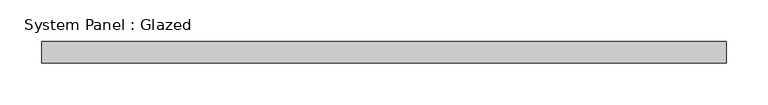
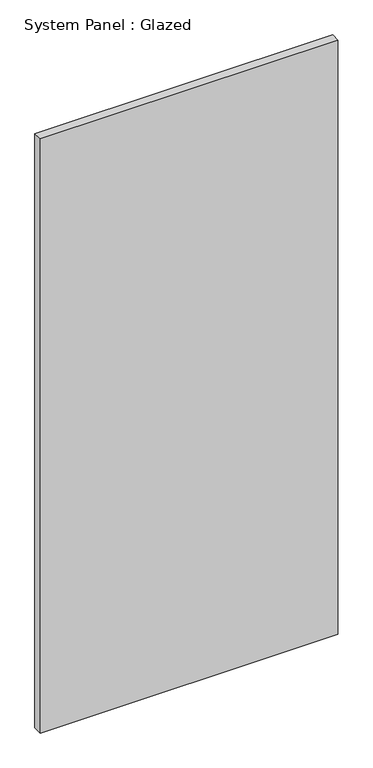
"""IFC4 building model written with IfcOpenShell, lengths in millimetres: plate geometry, System Panel : Glazed."""

from ifc_helpers import new_model, si_unit, origin, origin_with_axes, place, context, project, spatial, polyline, outline, extrude, source, transform, mapped, element, save


def system_panel_glazed_6affd56b(model_context):
    return source(origin(), model_context, "Body", "SweptSolid", [
        extrude(outline(polyline([(409.575, 19.05), (-409.575, 19.05), (-409.575, 44.45), (409.575, 44.45), (409.575, 19.05)])), origin_with_axes(), (0.0, 0.0, 1.0), 1728.6083676),
    ])


if __name__ == "__main__":
    model = new_model("IFC4")
    model_context = context("Model", 3, world=origin())
    ifc_project = project(units=[si_unit("LENGTHUNIT", "METRE", prefix="MILLI")], contexts=[model_context])
    site = spatial("IfcSite", under=ifc_project)
    building = spatial("IfcBuilding", under=site)
    placement = place(None, origin())
    system_panel_glazed_shape = system_panel_glazed_6affd56b(model_context)
    element("IfcPlate", 1, ObjectType="System Panel : Glazed", at=placement, inside=building, context=model_context, shape_type="MappedRepresentation", body=[
        mapped(system_panel_glazed_shape, transform((0.0, 0.0, 0.0), x_axis=(1.0, 0.0, 0.0), y_axis=(0.0, 1.0, 0.0), z_axis=(0.0, 0.0, 1.0))),
    ])
    save(model, "model.ifc")

# Revit data of these elements
# Type "System Panel : Glazed"
#   Construction Type Id = "GSP4R"
#   Analytic Construction = "1/8 in Pilkington single glazing"
#   Visual Light Transmittance = 0.9
#   Solar Heat Gain Coefficient = 0.86
#   Heat Transfer Coefficient (U) = 1.18115 BTU/(h·ft²·°F)
#   Define Thermal Properties by = 1
# Element 1 (IfcPlate, "System Panel : Glazed")
#   Materials on its faces: "Glass"
# Materials
#   "Glass": class "Glass", colour RGB 0 128 192, transparency 0.75, Description = "Soda Lime Glass", Cost = 0
